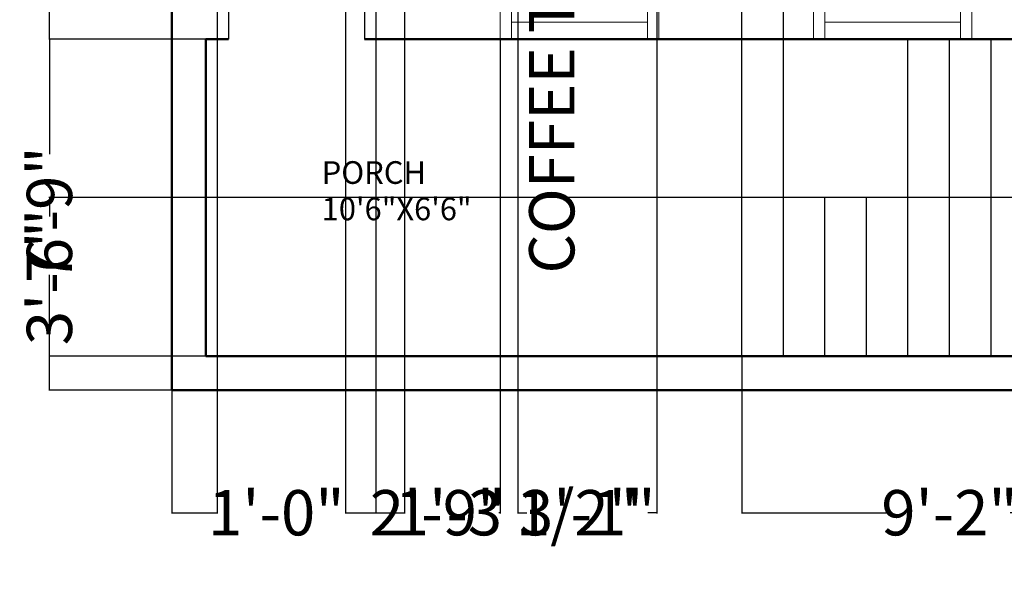
# Model space of a CAD drawing. Units: inches. Extents: x -51 to 1118, y -44 to 791.
# Tile 1 of 8: x -12 to 249, y -44 to 104. Entities that reach past the tile are written whole.
import ezdxf

# ---------------------------------------------------------------- set-up
doc = ezdxf.new("R2010")
doc.units = ezdxf.units.IN
doc.header["$MEASUREMENT"] = 0
for name, color, linetype, lineweight in [('A-ANNO-DIMS', 2, 'Continuous', 18), ('A-AREA-IDEN', 7, 'Continuous', 18), ('A-DOOR', 3, 'Continuous', 25), ('A-FLOR-STRS', 7, 'Continuous', 25), ('A-GLAZ', 4, 'Continuous', 18), ('A-WALL', 7, 'Continuous', 50)]:
    doc.layers.add(name, color=color, linetype=linetype, lineweight=lineweight)
doc.styles.get("Standard").update_dxf_attribs({"font": 'arial.ttf'})
doc.dimstyles.get("Standard").update_dxf_attribs({"dimtxt": 12, "dimasz": 0.18, "dimexe": 0.18, "dimexo": 0.0625, "dimgap": 0.09, "dimtad": 0, "dimdec": 1, "dimzin": 0, "dimdsep": 46, "dimlunit": 3, "dimtxsty": 'Standard', "dimcen": 0.09, "dimadec": 0, "dimazin": 0, "dimtfac": 1, "dimtdec": 1, "dimtofl": 0, "dimtmove": 0, "dimatfit": 3, "dimfxl": 1, "dimtolj": 1, "dimtzin": 0, "dimarcsym": 0})

# ---------------------------------------------------------------- blocks, each defined once
blk = doc.blocks.new('WIN-36IN')
for p, q in [((9, 42), (0, 42)), ((9, 39), (0, 39)), ((0, 39), (0, 3)), ((4.5, 3), (4.5, 39)), ((7.5, 3), (7.5, 39)), ((9, 3), (9, 39)), ((0, 3), (9, 3)), ((0, 0), (9, 0))]:
    blk.add_line(p, q)
blk = doc.blocks.new('DOOR-36IN-FRAME-9IN')
for p, q in [((0, 36.03), (0, 45.03)), ((3, 36.03), (3, 45.03)), ((39, 36.03), (39, 45.03)), ((42, 36.03), (42, 45.03))]:
    blk.add_line(p, q)
blk.add_lwpolyline([(39, 36.03), (36, 36.03), (36, 0.03), (39, 0.03)], close=True)
blk.add_arc((37.5, 34.53), 34.53, 177.5104, 272.4896)
blk = doc.blocks.new('*D28')
at = {"layer": 'A-ANNO-DIMS', "color": 0, "lineweight": -2, "transparency": 16777216}
for p, q in [((119.72, 254.44), (128.83, 254.44)), ((128.65, 254.26), (128.65, 194.62)), ((119.72, 194.44), (128.83, 194.44)), ((128.65, 194.44), (128.65, 194.26))]:
    blk.add_line(p, q, dxfattribs=at)
at = {"layer": 'A-ANNO-DIMS', "color": 0, "transparency": 16777216}
for points in [[(128.62, 254.26), (128.68, 254.26), (128.65, 254.44)], [(128.62, 194.62), (128.68, 194.62), (128.65, 194.44)]]:
    blk.add_solid(points, dxfattribs=at)
at = {"layer": 'Defpoints', "color": 0, "transparency": 16777216}
for p in [(119.65, 254.44), (119.65, 194.44), (128.65, 194.44)]:
    blk.add_point(p, dxfattribs=at)
at = {"layer": 'A-ANNO-DIMS', "color": 0, "transparency": 16777216, "insert": (128.65, 113.08), "char_height": 12, "attachment_point": 5, "rotation": 90}
blk.add_mtext('\\A1;COFFEE TABLE 5\'-0"', dxfattribs=at)
blk = doc.blocks.new('*D42')
at = {"layer": 'A-ANNO-DIMS', "color": 0, "lineweight": -2, "transparency": 16777216}
for p, q in [((36.96, 98.94), (-4.61, 98.94)), ((-4.43, 98.76), (-4.43, 68.43)), ((-4.43, 6.12), (-4.43, 36.45)), ((27.96, 5.94), (-4.61, 5.94))]:
    blk.add_line(p, q, dxfattribs=at)
at = {"layer": 'A-ANNO-DIMS', "color": 0, "transparency": 16777216}
for points in [[(-4.46, 98.76), (-4.4, 98.76), (-4.43, 98.94)], [(-4.46, 6.12), (-4.4, 6.12), (-4.43, 5.94)]]:
    blk.add_solid(points, dxfattribs=at)
at = {"layer": 'Defpoints', "color": 0, "transparency": 16777216}
for p in [(37.02, 98.94), (-4.43, 5.94), (28.02, 5.94)]:
    blk.add_point(p, dxfattribs=at)
at = {"layer": 'A-ANNO-DIMS', "color": 0, "transparency": 16777216, "insert": (-4.43, 52.44), "char_height": 12, "attachment_point": 5, "rotation": 90}
blk.add_mtext('\\A1;7\'-9"', dxfattribs=at)
blk = doc.blocks.new('*D44')
at = {"layer": 'A-ANNO-DIMS', "color": 0, "lineweight": -2, "transparency": 16777216}
for p, q in [((-4.43, 127.77), (-4.43, 127.95)), ((27.96, 127.77), (-4.61, 127.77)), ((-4.43, 99.12), (-4.43, 127.59)), ((36.96, 98.94), (-4.61, 98.94))]:
    blk.add_line(p, q, dxfattribs=at)
at = {"layer": 'A-ANNO-DIMS', "color": 0, "transparency": 16777216}
for points in [[(-4.46, 127.59), (-4.4, 127.59), (-4.43, 127.77)], [(-4.46, 99.12), (-4.4, 99.12), (-4.43, 98.94)]]:
    blk.add_solid(points, dxfattribs=at)
at = {"layer": 'Defpoints', "color": 0, "transparency": 16777216}
for p in [(-4.43, 127.77), (28.02, 127.77), (37.02, 98.94)]:
    blk.add_point(p, dxfattribs=at)
at = {"layer": 'A-ANNO-DIMS', "color": 0, "transparency": 16777216, "insert": (-4.43, 144.09), "char_height": 12, "attachment_point": 5, "rotation": 90}
blk.add_mtext('\\A1;2\'-5"', dxfattribs=at)
blk = doc.blocks.new('*D53')
at = {"layer": 'A-ANNO-DIMS', "color": 0, "lineweight": -2, "transparency": 16777216}
for p, q in [((40.02, 98.88), (40.02, -26.69)), ((28.02, 5.88), (28.02, -26.69)), ((28.2, -26.51), (39.84, -26.51)), ((40.02, -26.51), (40.2, -26.51))]:
    blk.add_line(p, q, dxfattribs=at)
at = {"layer": 'A-ANNO-DIMS', "color": 0, "transparency": 16777216}
for points in [[(28.2, -26.48), (28.2, -26.54), (28.02, -26.51)], [(39.84, -26.48), (39.84, -26.54), (40.02, -26.51)]]:
    blk.add_solid(points, dxfattribs=at)
at = {"layer": 'Defpoints', "color": 0, "transparency": 16777216}
for p in [(40.02, 98.94), (28.02, 5.94), (40.02, -26.51)]:
    blk.add_point(p, dxfattribs=at)
at = {"layer": 'A-ANNO-DIMS', "color": 0, "transparency": 16777216, "insert": (55.68, -26.51), "char_height": 12, "attachment_point": 5}
blk.add_mtext('\\A1;1\'-0"', dxfattribs=at)
blk = doc.blocks.new('*D54')
at = {"layer": 'A-ANNO-DIMS', "color": 0, "lineweight": -2, "transparency": 16777216}
for p, q in [((82.02, 98.88), (82.02, -26.69)), ((115.02, 98.88), (115.02, -26.69)), ((82.2, -26.51), (82.38, -26.51)), ((114.84, -26.51), (114.66, -26.51))]:
    blk.add_line(p, q, dxfattribs=at)
at = {"layer": 'A-ANNO-DIMS', "color": 0, "transparency": 16777216}
for points in [[(82.2, -26.48), (82.2, -26.54), (82.02, -26.51)], [(114.84, -26.48), (114.84, -26.54), (115.02, -26.51)]]:
    blk.add_solid(points, dxfattribs=at)
at = {"layer": 'Defpoints', "color": 0, "transparency": 16777216}
for p in [(82.02, 98.94), (115.02, 98.94), (115.02, -26.51)]:
    blk.add_point(p, dxfattribs=at)
at = {"layer": 'A-ANNO-DIMS', "color": 0, "transparency": 16777216, "insert": (98.52, -26.51), "char_height": 12, "attachment_point": 5}
blk.add_mtext('\\A1;2\'-9"', dxfattribs=at)
blk = doc.blocks.new('*D56')
at = {"layer": 'A-ANNO-DIMS', "color": 0, "lineweight": -2, "transparency": 16777216}
for p, q in [((178.96, 56.94), (-4.61, 56.94)), ((-4.43, 56.76), (-4.43, 51.98)), ((-4.43, 15.12), (-4.43, 19.9)), ((178.96, 14.94), (-4.61, 14.94))]:
    blk.add_line(p, q, dxfattribs=at)
at = {"layer": 'A-ANNO-DIMS', "color": 0, "transparency": 16777216}
for points in [[(-4.46, 56.76), (-4.4, 56.76), (-4.43, 56.94)], [(-4.46, 15.12), (-4.4, 15.12), (-4.43, 14.94)]]:
    blk.add_solid(points, dxfattribs=at)
at = {"layer": 'Defpoints', "color": 0, "transparency": 16777216}
for p in [(-4.43, 56.94), (179.02, 56.94), (179.02, 14.94)]:
    blk.add_point(p, dxfattribs=at)
at = {"layer": 'A-ANNO-DIMS', "color": 0, "transparency": 16777216, "insert": (-4.43, 35.94), "char_height": 12, "attachment_point": 5, "rotation": 90}
blk.add_mtext('\\A1;3\'-6"', dxfattribs=at)
blk = doc.blocks.new('*D57')
at = {"layer": 'A-ANNO-DIMS', "color": 0, "lineweight": -2, "transparency": 16777216}
for p, q in [((179.02, 57), (179.02, 638.57)), ((179.2, 638.39), (189.84, 638.39)), ((190.02, 57), (190.02, 638.57)), ((190.02, 638.39), (190.2, 638.39))]:
    blk.add_line(p, q, dxfattribs=at)
at = {"layer": 'A-ANNO-DIMS', "color": 0, "transparency": 16777216}
for points in [[(179.2, 638.42), (179.2, 638.36), (179.02, 638.39)], [(189.84, 638.42), (189.84, 638.36), (190.02, 638.39)]]:
    blk.add_solid(points, dxfattribs=at)
at = {"layer": 'Defpoints', "color": 0, "transparency": 16777216}
for p in [(190.02, 638.39), (179.02, 56.94), (190.02, 56.94)]:
    blk.add_point(p, dxfattribs=at)
at = {"layer": 'A-ANNO-DIMS', "color": 0, "transparency": 16777216, "insert": (210.9, 638.39), "char_height": 12, "attachment_point": 5}
blk.add_mtext('\\A1;0\'-11"', dxfattribs=at)
blk = doc.blocks.new('*D58')
at = {"layer": 'A-ANNO-DIMS', "color": 0, "lineweight": -2, "transparency": 16777216}
for p, q in [((179.02, 14.88), (179.02, -26.69)), ((289.02, 14.88), (289.02, -26.69)), ((179.2, -26.51), (217.98, -26.51)), ((288.84, -26.51), (250.06, -26.51))]:
    blk.add_line(p, q, dxfattribs=at)
at = {"layer": 'A-ANNO-DIMS', "color": 0, "transparency": 16777216}
for points in [[(179.2, -26.48), (179.2, -26.54), (179.02, -26.51)], [(288.84, -26.48), (288.84, -26.54), (289.02, -26.51)]]:
    blk.add_solid(points, dxfattribs=at)
at = {"layer": 'Defpoints', "color": 0, "transparency": 16777216}
for p in [(179.02, 14.94), (289.02, 14.94), (179.02, -26.51)]:
    blk.add_point(p, dxfattribs=at)
at = {"layer": 'A-ANNO-DIMS', "color": 0, "transparency": 16777216, "insert": (234.02, -26.51), "char_height": 12, "attachment_point": 5}
blk.add_mtext('\\A1;9\'-2"', dxfattribs=at)
blk = doc.blocks.new('*D59')
at = {"layer": 'A-ANNO-DIMS', "color": 0, "lineweight": -2, "transparency": 16777216}
for p, q in [((89.65, 194.38), (89.65, -26.69)), ((74, 189.63), (74, -26.69)), ((74.18, -26.51), (89.47, -26.51)), ((89.65, -26.51), (89.83, -26.51))]:
    blk.add_line(p, q, dxfattribs=at)
at = {"layer": 'A-ANNO-DIMS', "color": 0, "transparency": 16777216}
for points in [[(74.18, -26.48), (74.18, -26.54), (74, -26.51)], [(89.47, -26.48), (89.47, -26.54), (89.65, -26.51)]]:
    blk.add_solid(points, dxfattribs=at)
at = {"layer": 'Defpoints', "color": 0, "transparency": 16777216}
for p in [(89.65, 194.44), (74, 189.69), (89.65, -26.51)]:
    blk.add_point(p, dxfattribs=at)
at = {"layer": 'A-ANNO-DIMS', "color": 0, "transparency": 16777216, "insert": (119.29, -26.51), "char_height": 12, "attachment_point": 5}
blk.add_mtext('\\A1;1\'-3 1/2"', dxfattribs=at)
blk = doc.blocks.new('*D60')
at = {"layer": 'A-ANNO-DIMS', "color": 0, "lineweight": -2, "transparency": 16777216}
for p, q in [((119.65, 194.38), (119.65, -26.69)), ((156.48, 194.05), (156.48, -26.69)), ((119.83, -26.51), (122.03, -26.51)), ((156.3, -26.51), (154.1, -26.51))]:
    blk.add_line(p, q, dxfattribs=at)
at = {"layer": 'A-ANNO-DIMS', "color": 0, "transparency": 16777216}
for points in [[(119.83, -26.48), (119.83, -26.54), (119.65, -26.51)], [(156.3, -26.48), (156.3, -26.54), (156.48, -26.51)]]:
    blk.add_solid(points, dxfattribs=at)
at = {"layer": 'Defpoints', "color": 0, "transparency": 16777216}
for p in [(119.65, 194.44), (156.48, 194.11), (156.48, -26.51)]:
    blk.add_point(p, dxfattribs=at)
at = {"layer": 'A-ANNO-DIMS', "color": 0, "transparency": 16777216, "insert": (138.06, -26.51), "char_height": 12, "attachment_point": 5}
blk.add_mtext('\\A1;3\'-1"', dxfattribs=at)

msp = doc.modelspace()

# ---------------------------------------------------------------- linework, layer by layer
at = {"layer": 'A-FLOR-STRS'}
for p, q in [((223.02, 14.94), (223.02, 98.94)), ((234.02, 14.94), (234.02, 98.94)), ((245.02, 14.94), (245.02, 98.94)), ((179.02, 14.94), (179.02, 56.94)), ((289.02, 56.94), (179.02, 56.94)), ((190.02, 14.94), (190.02, 56.94)), ((201.02, 14.94), (201.02, 56.94)), ((212.02, 14.94), (212.02, 56.94))]:
    msp.add_line(p, q, dxfattribs=at)
at = {"layer": 'A-WALL'}
for p, q in [((37.02, 98.94), (37.02, 14.94)), ((43.02, 98.94), (37.02, 98.94)), ((331.02, 98.94), (79.02, 98.94)), ((37.02, 14.94), (331.02, 14.94))]:
    msp.add_line(p, q, dxfattribs=at)
msp.add_lwpolyline([(145.02, 605.94), (28.02, 605.94), (28.02, 5.94), (340.02, 5.94), (340.02, 605.94), (181.02, 605.94)], dxfattribs=at)

# ---------------------------------------------------------------- block references
at = {"layer": 'A-DOOR', "rotation": 180}
msp.add_blockref('DOOR-36IN-FRAME-9IN', (82.02, 143.97), dxfattribs=at)
at = {"layer": 'A-GLAZ'}
for p, rotation in [((157.02, 98.94), 90.00000000000003), ((239.97, 98.94), 89.99999999999996)]:
    msp.add_blockref('WIN-36IN', p, dxfattribs=dict(at, rotation=rotation))

# ---------------------------------------------------------------- texts
at = {"layer": 'A-AREA-IDEN'}
for s, p in [('PORCH', (67.7, 60.58)), ('10\'6"X6\'6"', (67.7, 50.94))]:
    msp.add_text(s, height=6, dxfattribs=at).set_placement(p)

# ---------------------------------------------------------------- dimensions: what is measured, and where the dimension line sits
at = {"layer": 'A-ANNO-DIMS'}
for base, p1, p2, picture, middle in [((190.02, 638.39), (179.02, 56.94), (190.02, 56.94), '*D57', (210.9, 638.39)), ((89.6538, -26.5097), (74.0019, 189.6882), (89.6538, 194.4401), '*D59', (119.2895, -26.5097)), ((156.48, -26.51), (119.65, 194.44), (156.48, 194.11), '*D60', (138.06, -26.51)), ((40.02, -26.51), (28.02, 5.94), (40.02, 98.94), '*D53', (55.68, -26.51)), ((115.02, -26.51), (82.02, 98.94), (115.02, 98.94), '*D54', (98.52, -26.51)), ((179.02, -26.51), (289.02, 14.94), (179.02, 14.94), '*D58', (234.02, -26.51))]:
    dim = msp.add_linear_dim(base=base, p1=p1, p2=p2, dimstyle='Standard', override={"dimdec": 1, "dimlfac": 1, "dimrnd": 0, "dimzin": 1, "dimdsep": 46, "dimlunit": 4, "dimfrac": 2}, dxfattribs=at)
    dim.commit()
    dim.dimension.update_dxf_attribs({"geometry": picture, "text_midpoint": middle})
dim = msp.add_linear_dim(base=(128.65, 194.44), p1=(119.65, 254.44), p2=(119.65, 194.44), angle=270, text='COFFEE TABLE <>', dimstyle='Standard', override={"dimdec": 1, "dimlfac": 1, "dimrnd": 0, "dimzin": 1, "dimdsep": 46, "dimlunit": 4, "dimfrac": 2}, dxfattribs=at)
dim.commit()
dim.dimension.update_dxf_attribs({"geometry": '*D28', "text_midpoint": (128.65, 113.08)})
for base, p1, p2, picture, middle in [((-4.43, 127.77), (37.02, 98.94), (28.02, 127.77), '*D44', (-4.43, 144.09)), ((-4.43, 5.94), (37.02, 98.94), (28.02, 5.94), '*D42', (-4.43, 52.44)), ((-4.43, 56.94), (179.02, 14.94), (179.02, 56.94), '*D56', (-4.43, 35.94))]:
    dim = msp.add_linear_dim(base=base, p1=p1, p2=p2, angle=90, dimstyle='Standard', override={"dimdec": 1, "dimlfac": 1, "dimrnd": 0, "dimzin": 1, "dimdsep": 46, "dimlunit": 4, "dimfrac": 2}, dxfattribs=at)
    dim.commit()
    dim.dimension.update_dxf_attribs({"geometry": picture, "text_midpoint": middle})

doc.saveas('drawing.dxf')
